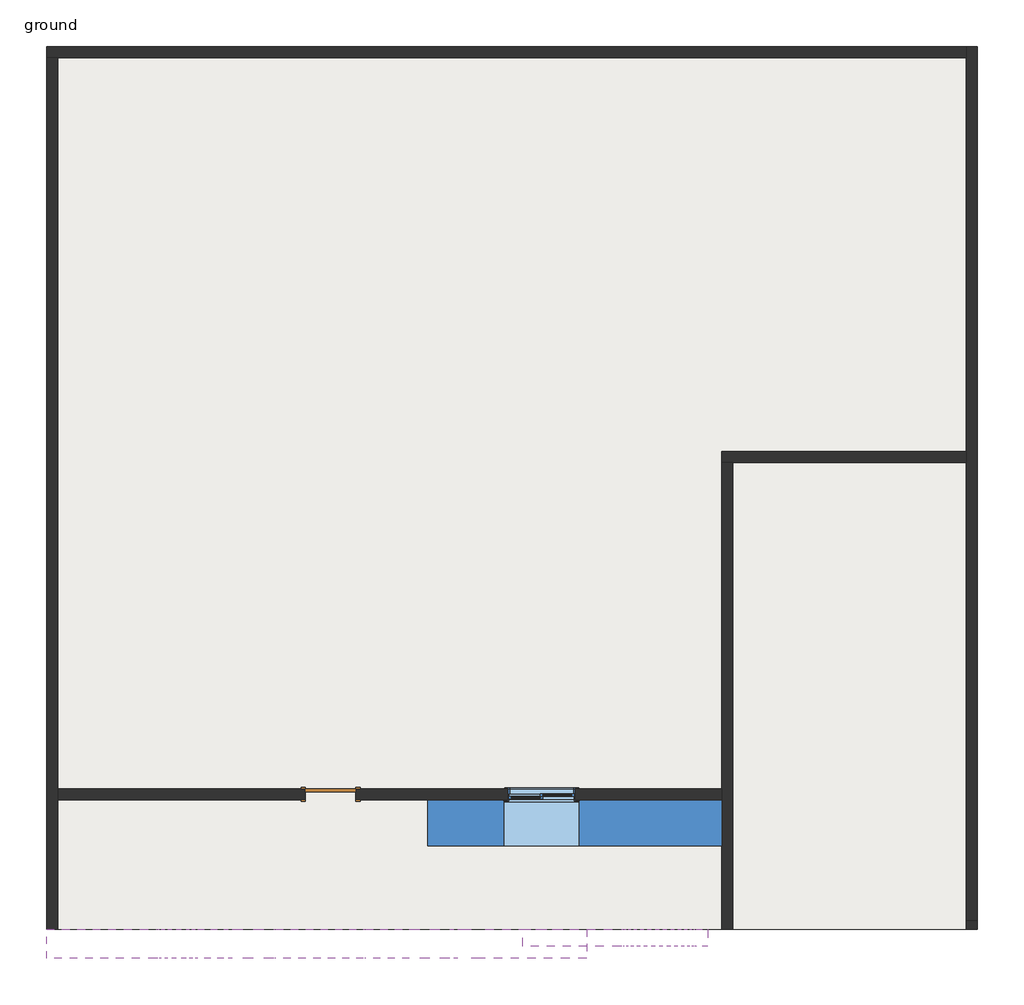
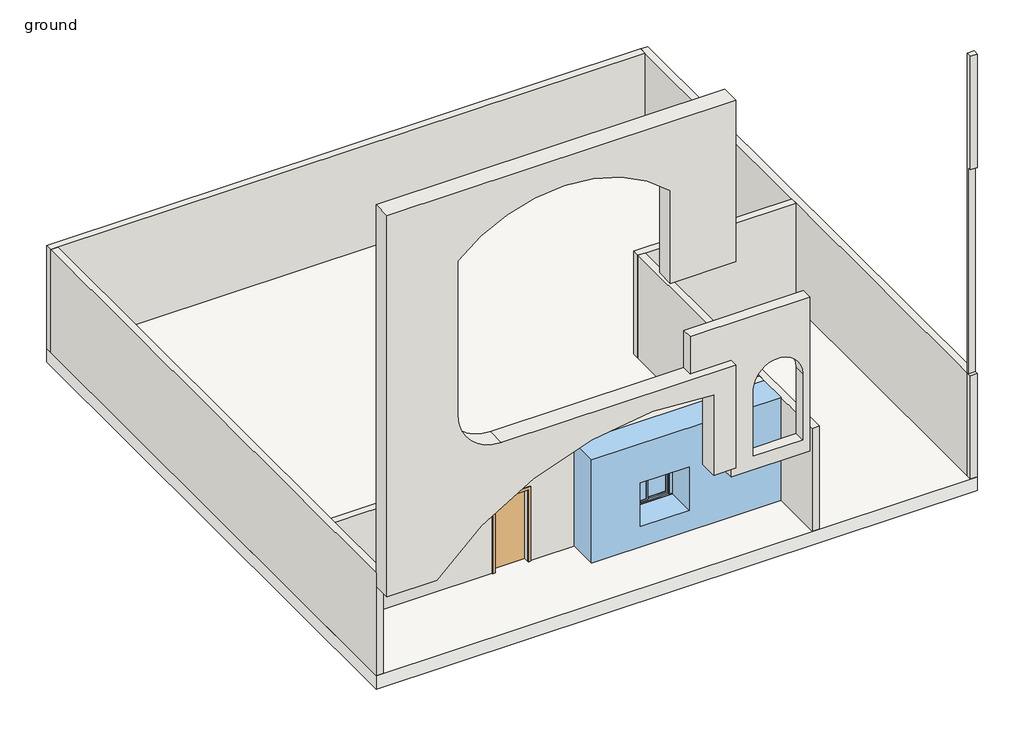
# One storey: 9 walls, 2 windows, 1 door, 1 slab.
"""IFC4 building model written with IfcOpenShell, lengths in millimetres."""

from ifc_helpers import new_model, si_unit, frame, origin, place, context, project, spatial, polyline, outline, extrude, faceted_brep, transform, mapped, element, save
from components import m_single_flush_0915_x_2134mm_727434cd, walls_1_walls_1_8e9adab5, walls_2_walls_2_f3eab2de, window_deda82dd, windows_1_windows_1_29d15952

model = new_model("IFC4")

# Units and contexts
model_context = context("Model", 3, world=origin())
ifc_project = project(units=[si_unit("LENGTHUNIT", "METRE", prefix="MILLI")], contexts=[model_context])

# Site, building, storey
site = spatial("IfcSite", under=ifc_project)
building = spatial("IfcBuilding", under=site)
storey = spatial("IfcBuildingStorey", under=building, Name="ground", Elevation=0.0)

# Door
placement = place(None, origin())
m_single_flush_0915_x_2134mm_shape = m_single_flush_0915_x_2134mm_727434cd(model_context)
element("IfcDoor", 1, ObjectType="M_Single-Flush : 0915 x 2134mm", at=placement, inside=storey, context=model_context, shape_type="MappedRepresentation", body=[
    mapped(m_single_flush_0915_x_2134mm_shape, transform((-3902.6352527, 1849.2148445, 0.0), x_axis=(-1.0, 0.0, 0.0), y_axis=(0.0, -1.0, 0.0), z_axis=(0.0, 0.0, 1.0))),
])

# Slab
element("IfcSlab", 2, ObjectType="Generic Floor - 400mm", at=placement, inside=storey, context=model_context, shape_type="SweptSolid", body=[
    extrude(outline(polyline([(-9031.8352527, 15360.4148445), (7778.3159626, 15360.4148445), (7778.3159626, -589.1851555), (-9031.8352527, -589.1851555), (-9031.8352527, 15360.4148445)])), frame((0.0, 0.0, -400.0), z_axis=(0.0, 0.0, 1.0), x_axis=(1.0, 0.0, 0.0)), (0.0, 0.0, 1.0), 400.0),
])

# Walls
element("IfcWall", 3, ObjectType="Generic - 9\"", at=placement, inside=storey, context=model_context, shape_type="Brep", body=[
    faceted_brep([(-9031.8352527, 15160.4148445, 0.0), (-8831.8352527, 15160.4148445, 0.0), (7578.3159626, 15160.4148445, 0.0), (7578.3159626, 15160.4148445, 3048.0), (-8831.8352527, 15160.4148445, 3048.0), (-9031.8352527, 15160.4148445, 3048.0), (-9031.8352527, 15360.4148445, 0.0), (-9031.8352527, 15360.4148445, 3048.0), (7578.3159626, 15360.4148445, 3048.0), (7578.3159626, 15360.4148445, 0.0)], [[[0, 1, 2, 3, 4, 5]], [[6, 7, 8, 9]], [[2, 1, 0, 6, 9]], [[5, 4, 3, 8, 7]], [[0, 5, 7, 6]], [[3, 2, 9, 8]]]),
])
element("IfcWall", 4, ObjectType="Generic - 9\"", at=placement, inside=storey, context=model_context, shape_type="Brep", body=[
    faceted_brep([(-8831.8352527, -589.1851555, 0.0), (-8831.8352527, 1749.2148445, 0.0), (-8831.8352527, 1949.2148445, 0.0), (-8831.8352527, 15160.4148445, 0.0), (-8831.8352527, 15160.4148445, 3048.0), (-8831.8352527, 1949.2148445, 3048.0), (-8831.8352527, 1749.2148445, 3048.0), (-8831.8352527, -589.1851555, 3048.0), (-9031.8352527, -589.1851555, 0.0), (-9031.8352527, -589.1851555, 3048.0), (-9031.8352527, 15160.4148445, 3048.0), (-9031.8352527, 15160.4148445, 0.0)], [[[0, 1, 2, 3, 4, 5, 6, 7]], [[8, 9, 10, 11]], [[3, 2, 1, 0, 8, 11]], [[7, 6, 5, 4, 10, 9]], [[0, 7, 9, 8]], [[4, 3, 11, 10]]]),
])
element("IfcWall", 5, ObjectType="Generic - 9\"", at=placement, inside=storey, context=model_context, shape_type="Brep", body=[
    faceted_brep([(7578.3159626, 15360.4148445, 0.0), (7578.3159626, 15160.4148445, 0.0), (7578.3159626, 8045.2148445, 0.0), (7578.3159626, 7845.2148445, 0.0), (7578.3159626, -589.1851555, 0.0), (7578.3159626, -589.1851555, 3048.0), (7578.3159626, 7845.2148445, 3048.0), (7578.3159626, 8045.2148445, 3048.0), (7578.3159626, 15160.4148445, 3048.0), (7578.3159626, 15360.4148445, 3048.0), (7778.3159626, 15360.4148445, 0.0), (7778.3159626, 15360.4148445, 3048.0), (7778.3159626, -589.1851555, 3048.0), (7778.3159626, -589.1851555, 0.0)], [[[0, 1, 2, 3, 4, 5, 6, 7, 8, 9]], [[10, 11, 12, 13]], [[4, 3, 2, 1, 0, 10, 13]], [[5, 4, 13, 12]], [[9, 8, 7, 6, 5, 12, 11]], [[0, 9, 11, 10]]]),
])
element("IfcWall", 6, ObjectType="Generic - 9\"", at=placement, inside=storey, context=model_context, shape_type="Brep", body=[
    faceted_brep([(3160.1647473, 7845.2148445, 0.0), (3360.1647473, 7845.2148445, 0.0), (7578.3159626, 7845.2148445, 0.0), (7578.3159626, 7845.2148445, 3048.0), (3360.1647473, 7845.2148445, 3048.0), (3160.1647473, 7845.2148445, 3048.0), (3160.1647473, 8045.2148445, 0.0), (3160.1647473, 8045.2148445, 3048.0), (7578.3159626, 8045.2148445, 3048.0), (7578.3159626, 8045.2148445, 0.0)], [[[0, 1, 2, 3, 4, 5]], [[6, 7, 8, 9]], [[2, 1, 0, 6, 9]], [[5, 4, 3, 8, 7]], [[0, 5, 7, 6]], [[3, 2, 9, 8]]]),
])
element("IfcWall", 7, ObjectType="Generic - 9\"", at=placement, inside=storey, context=model_context, shape_type="Brep", body=[
    faceted_brep([(3360.1647473, -589.1851555, 0.0), (3360.1647473, 7845.2148445, 0.0), (3360.1647473, 7845.2148445, 3048.0), (3360.1647473, -589.1851555, 3048.0), (3160.1647473, -589.1851555, 0.0), (3160.1647473, -589.1851555, 3048.0), (3160.1647473, 1749.2148445, 3048.0), (3160.1647473, 1949.2148445, 3048.0), (3160.1647473, 7845.2148445, 3048.0), (3160.1647473, 7845.2148445, 0.0), (3160.1647473, 1949.2148445, 0.0), (3160.1647473, 1749.2148445, 0.0)], [[[0, 1, 2, 3]], [[4, 5, 6, 7, 8, 9, 10, 11]], [[1, 0, 4, 11, 10, 9]], [[3, 2, 8, 7, 6, 5]], [[0, 3, 5, 4]], [[2, 1, 9, 8]]]),
])
element("IfcWall", 8, ObjectType="Generic - 9\"", at=placement, inside=storey, context=model_context, shape_type="SweptSolid", body=[
    extrude(outline(polyline([(0.0, -8831.8352527), (0.0, -4360.1352527), (2134.0, -4360.1352527), (2134.0, -3445.1352527), (0.0, -3445.1352527), (0.0, 3160.1647473), (3048.0, 3160.1647473), (3048.0, -8831.8352527), (0.0, -8831.8352527)]), holes=[polyline([(1828.8, -702.2352527), (1828.8, 516.9647473), (609.6, 516.9647473), (609.6, -702.2352527), (1828.8, -702.2352527)])]), frame((0.0, 1749.2148445, 0.0), z_axis=(0.0, 1.0, 0.0), x_axis=(0.0, 0.0, 1.0)), (0.0, 0.0, 1.0), 200.0),
])
element("IfcWall", 9, ObjectType="Generic - 9\"", at=placement, inside=storey, context=model_context, shape_type="SweptSolid", body=[
    extrude(outline(polyline([(-589.1851555, 0.0), (-589.1851555, 3048.0), (-489.1851555, 3048.0), (-489.1851555, 9144.0), (-589.1851555, 9144.0), (-589.1851555, 12496.8), (-436.7851555, 12496.8), (-436.7851555, 0.0), (-589.1851555, 0.0)])), frame((7578.3159626, 0.0, 0.0), z_axis=(1.0, 0.0, 0.0), x_axis=(0.0, 1.0, 0.0)), (0.0, 0.0, 1.0), 200.0),
])
walls_1_walls_1_shape = walls_1_walls_1_8e9adab5(model_context)
element("IfcWall", 10, ObjectType="Walls 1 : Walls 1", at=placement, inside=storey, context=model_context, shape_type="MappedRepresentation", body=[
    mapped(walls_1_walls_1_shape, transform((0.0, 0.0, 0.0), x_axis=(1.0, 0.0, 0.0), y_axis=(0.0, 1.0, 0.0), z_axis=(0.0, 0.0, 1.0))),
])
walls_2_walls_2_shape = walls_2_walls_2_f3eab2de(model_context)
element("IfcWall", 11, ObjectType="Walls 2 : Walls 2", at=placement, inside=storey, context=model_context, shape_type="MappedRepresentation", body=[
    mapped(walls_2_walls_2_shape, transform((0.0, 0.0, 0.0), x_axis=(1.0, 0.0, 0.0), y_axis=(0.0, 1.0, 0.0), z_axis=(0.0, 0.0, 1.0))),
])

# Windows
window_shape = window_deda82dd(model_context)
element("IfcWindow", 12, ObjectType="Slider with Trim : 48\" x 48\"", at=placement, inside=storey, context=model_context, shape_type="MappedRepresentation", body=[
    mapped(window_shape, transform((-92.6352527, 1849.2148445, -304.8), x_axis=(-1.0, 0.0, 0.0), y_axis=(0.0, -1.0, 0.0), z_axis=(0.0, 0.0, 1.0))),
])
windows_1_windows_1_shape = windows_1_windows_1_29d15952(model_context)
element("IfcWindow", 13, ObjectType="Windows 1 : Windows 1", at=placement, inside=storey, context=model_context, shape_type="MappedRepresentation", body=[
    mapped(windows_1_windows_1_shape, transform((0.0, 0.0, 0.0), x_axis=(1.0, 0.0, 0.0), y_axis=(0.0, 1.0, 0.0), z_axis=(0.0, 0.0, 1.0))),
])

save(model, "model.ifc")

# Revit data of these elements
# Type "M_Single-Flush : 0915 x 2134mm"
#   Type Mark = "15"
#   Thickness = 0' - 2.00787"
#   Height = 7' - 0.01575"
#   Trim Projection Ext = 0' - 0.98425"
#   Trim Projection Int = 0' - 0.98425"
#   Trim Width = 0' - 2.99213"
#   Width = 3' - 0.02362"
#   Door Material = Door - Panel
#   Frame Material = Door - Frame
#   Function = (empty or 0)
#   Wall Closure = (empty or 0)
# Type "Generic Floor - 400mm"
#   Function = 0
#   Layers, outside or top first: 1' - 3.74803" no material (function 1)
# Type "Generic - 9\""
#   Layers, outside or top first: 0' - 7.87402" no material (function 1)
# Type "Slider with Trim : 48\" x 48\""
#   Type Mark = "24"
#   Construction Type Id = "GSP4R"
#   Assembly Code = "B2020100"
#   Analytic Construction = "1/8 in Pilkington single glazing"
#   Visual Light Transmittance = 0.9
#   Solar Heat Gain Coefficient = 0.78
#   Heat Transfer Coefficient (U) = 3.6886 W/(m²·K)
#   Height = 4' - 0"
#   Default Sill Height = 3' - 0"
#   Trim Projection - Ext. = 0' - 0 3/4"
#   Trim Projection - Int. = 0' - 0 3/4"
#   Trim Width - Exterior = 0' - 3 1/2"
#   Trim Width - Interior = 0' - 3 1/2"
#   Width = 4' - 0"
#   Window Inset = 0' - 0 3/4"
#   Define Thermal Properties by = 1
#   Glass Pane Material = Glass
#   Sash Material = Sash
#   Trim Exterior Material = Trim
#   Trim Interior Material = Trim
#   Wall Closure = (empty or 0)
# Type "Windows 1 : Windows 1"
#   Type Mark = "25"
# Element 1 (IfcDoor, "M_Single-Flush : 0915 x 2134mm")
#   Phase Created = New Construction
#   Materials on its faces: "Door - Frame", "Door - Panel"
# Element 2 (IfcSlab, "Generic Floor - 400mm")
#   built-in parameter 1001955 = 3.14159 (stored number, unit not read)
#   Height Offset From Level = 0' - 0"
#   Phase Created = New Construction
#   Materials on its faces: "Default Roof"
# Elements 3, 4, 5, 6, 7, 8 (IfcWall, "Generic - 9\"")
#   Top Offset = 0' - 0"
#   Base Offset = 0' - 0"
#   Unconnected Height = 10' - 0"
#   wall height = 10' - 0"
#   Phase Created = New Construction
#   Base Constraint = ground
#   Materials on its faces: "Default Wall"
# Element 9 (IfcWall, "Generic - 9\"")
#   Top Offset = 0' - 0"
#   Base Offset = 0' - 0"
#   Unconnected Height = 41' - 0"
#   wall height = 41' - 0"
#   Phase Created = New Construction
#   Base Constraint = ground
#   Materials on its faces: "Default Wall"
# Element 10 (IfcWall, "Walls 1 : Walls 1")
#   Phase Created = New Construction
#   Materials on its faces: "Default Wall"
# Element 11 (IfcWall, "Walls 2 : Walls 2")
#   Phase Created = New Construction
#   Materials on its faces: "Default Wall"
# Element 12 (IfcWindow, "Slider with Trim : 48\" x 48\"")
#   Mark = "6"
#   Phase Created = New Construction
#   Materials on its faces: "Sash", "Trim", "Glass"
# Element 13 (IfcWindow, "Windows 1 : Windows 1")
#   Mark = "7"
#   Phase Created = New Construction
# Materials
#   "Door - Panel": class "Wood", colour RGB 114 82 51, transparency 0
#   "Door - Frame": colour RGB 153 76 43, transparency 0
#   "Glass": class "Glass", colour RGB 218 227 224, transparency 0.85, Description = "Soda Lime Glass", Cost = 0
#   "Sash": class "Wood", colour RGB 136 99 55, transparency 0
#   "Trim": class "Wood", colour RGB 224 178 126, transparency 0
#   "Default Roof": colour RGB 80 80 80, transparency 0
#   "Default Wall": colour RGB 80 80 80, transparency 0
